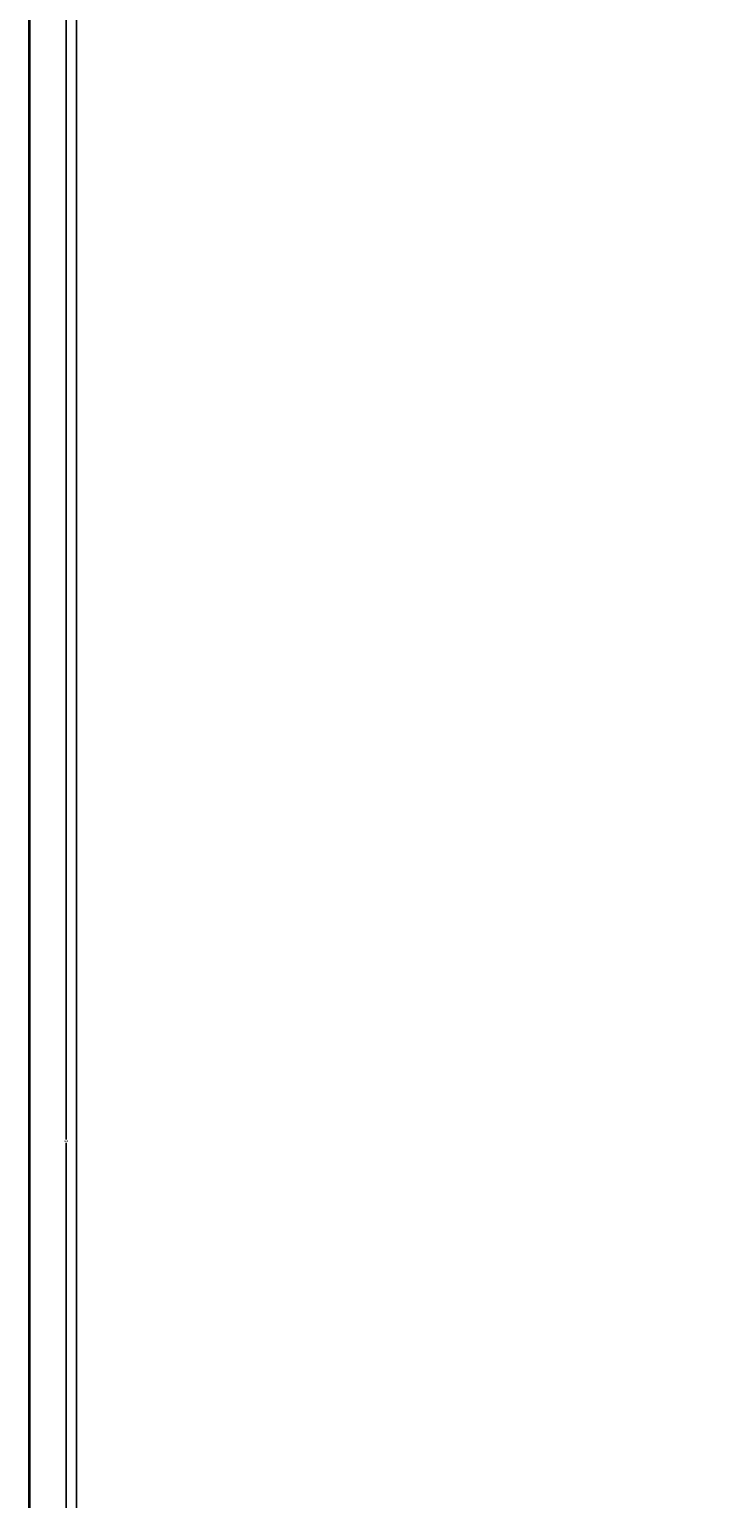
# Model space of a CAD drawing. Units: inches. Extents: x 1602 to 2642, y 1463 to 2270.
# Tile 3 of 5: x 2039 to 2113, y 1763 to 1919. Entities that reach past the tile are written whole.
import ezdxf

# ---------------------------------------------------------------- set-up
doc = ezdxf.new("R2010")
doc.units = ezdxf.units.IN
for name, color, linetype, lineweight in [('A-ANNO-DIMS', 2, 'Continuous', 18), ('A-WALL', 7, 'Continuous', 35), ('C-PROP', 7, 'Continuous', 25)]:
    doc.layers.add(name, color=color, linetype=linetype, lineweight=lineweight)
doc.styles.get("Standard").update_dxf_attribs({"font": 'arial.ttf'})
doc.dimstyles.get("Standard").update_dxf_attribs({"dimtxt": 0.18, "dimasz": 0.18, "dimexe": 0.18, "dimexo": 0.0625, "dimgap": 0.09, "dimtad": 0, "dimtih": 1, "dimtoh": 1, "dimdec": 4, "dimzin": 0, "dimdsep": 46, "dimtxsty": 'Standard', "dimcen": 0.09, "dimadec": 0, "dimazin": 0, "dimtfac": 1, "dimtdec": 4, "dimtofl": 0, "dimtmove": 0, "dimatfit": 3, "dimfxl": 1, "dimtolj": 1, "dimtzin": 0, "dimarcsym": 0})

# ---------------------------------------------------------------- blocks, each defined once
blk = doc.blocks.new('*D42')
at = {"layer": 'A-ANNO-DIMS', "color": 0, "lineweight": -2, "transparency": 16777216}
for p, q in [((2130.593932000001, 2100.748103000001), (2042.459860000002, 2100.748103000001)), ((2042.639860000002, 2100.568103000001), (2042.639860000002, 1800.930006137791)), ((2042.639860000002, 1500.928103), (2042.639860000002, 1800.566199862211)), ((2130.593932000001, 1500.748103), (2042.459860000002, 1500.748103))]:
    blk.add_line(p, q, dxfattribs=at)
at = {"layer": 'A-ANNO-DIMS', "color": 0, "transparency": 16777216}
for points in [[(2042.609860000002, 2100.568103000001), (2042.669860000002, 2100.568103000001), (2042.639860000002, 2100.748103000001)], [(2042.609860000002, 1500.928103), (2042.669860000002, 1500.928103), (2042.639860000002, 1500.748103)]]:
    blk.add_solid(points, dxfattribs=at)
at = {"layer": 'Defpoints', "color": 0, "transparency": 16777216}
for p in [(2042.639860000002, 2100.748103000001), (2130.656432000001, 2100.748103000001), (2130.656432000001, 1500.748103)]:
    blk.add_point(p, dxfattribs=at)
at = {"layer": 'A-ANNO-DIMS', "color": 0, "transparency": 16777216, "insert": (2042.639860000002, 1800.748103), "char_height": 0.18, "attachment_point": 5}
blk.add_mtext('\\A1;600', dxfattribs=at)

msp = doc.modelspace()

# ---------------------------------------------------------------- linework, layer by layer
at = {"layer": 'A-WALL'}
msp.add_line((2038.726933683589, 1734.248102623292), (2038.726933683589, 2100.748102623293), dxfattribs=at)
at = {"layer": 'C-PROP'}
msp.add_line((2043.726933683589, 1500.748102623292), (2043.726933683589, 2100.748102623293), dxfattribs=at)

# ---------------------------------------------------------------- dimensions: what is measured, and where the dimension line sits
at = {"layer": 'A-ANNO-DIMS'}
dim = msp.add_linear_dim(base=(2042.639860000002, 2100.748103000001), p1=(2130.656432, 1500.748103), p2=(2130.656432, 2100.748103), angle=90, dimstyle='Standard', override={"dimdec": 0, "dimlfac": 1, "dimrnd": 0, "dimzin": 0, "dimdsep": 46, "dimlunit": 2}, dxfattribs=at)
dim.commit()
dim.dimension.update_dxf_attribs({"geometry": '*D42', "text_midpoint": (2042.639860000002, 1800.748103)})

doc.saveas('drawing.dxf')
